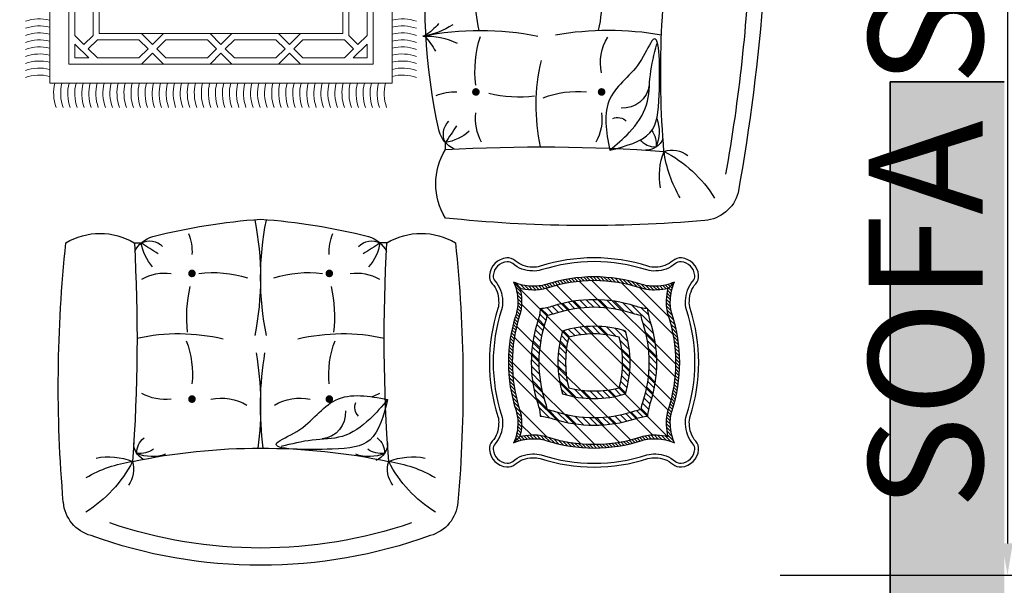
# Model space of a CAD drawing. Units: inches. Extents: x 3592 to 4861, y 1650 to 2243.
# Tile 5 of 30: x 4188 to 4265, y 1872 to 1916. Entities that reach past the tile are written whole.
import ezdxf

# ---------------------------------------------------------------- set-up
doc = ezdxf.new("R2010")
doc.units = ezdxf.units.IN
for name, color, linetype, lineweight in [('A-ANNO-DIMS', 2, 'Continuous', 13), ('A-FURN', 9, 'Continuous', 13), ('A-WALL', 7, 'Continuous', 35), ('RA-AP-01$0$INT', 35, 'Continuous', 5)]:
    doc.layers.add(name, color=color, linetype=linetype, lineweight=lineweight)
doc.layers.add('A-WALL-PATT', color=252, linetype='Continuous', lineweight=13, true_color=0x939598)
for name, color, linetype in [('RA-AP-01$0$FURN', 3, 'Continuous'), ('RA-AP-01$0$WOOD', 64, 'Continuous'), ('RA-AP-02$0$FLPT', 30, 'Continuous')]:
    doc.layers.add(name, color=color, linetype=linetype)
doc.styles.get("Standard").update_dxf_attribs({"font": 'arial.ttf'})
doc.dimstyles.new('ISO-25', dxfattribs={"dimtxt": 9, "dimasz": 2.5, "dimexe": 1.25, "dimexo": 0.625, "dimtad": 1, "dimlunit": 3, "dimtxsty": 'Standard', "dimcen": 2.5, "dimadec": 0, "dimazin": 0, "dimtfac": 1, "dimtmove": 0, "dimatfit": 3, "dimfxl": 1, "dimarcsym": 0})
pattern_1 = [(225, (10.907943, -14.206733), (0.008838835, -0.008838835), [])]
pattern_2 = [(225, (10.9079426, -14.206733), (0.0044194174, -0.0044194174), [])]

# ---------------------------------------------------------------- blocks, each defined once
blk = doc.blocks.new('A$C7F4351E2')
at = {"layer": 'RA-AP-01$0$FURN'}
for p, q in [((8.3526, -8.2639), (8.3526, -8.2823)), ((8.3526, -8.9277), (8.3526, -8.9094))]:
    blk.add_line(p, q, dxfattribs=at)
at = {"layer": 'RA-AP-01$0$FURN', "const_width": 0.01}
for points in [[(8.4378, -8.4154, 1), (8.4278, -8.4154, 1)], [(8.7582, -8.4154, -1), (8.7682, -8.4154, -1)], [(8.4378, -8.7763, -1), (8.4278, -8.7763, -1)], [(8.7582, -8.7763, 1), (8.7682, -8.7763, 1)]]:
    blk.add_lwpolyline(points, format="xyb", close=True, dxfattribs=at)
at = {"layer": 'RA-AP-01$0$FURN'}
for centre, radius, start, end in [((8.7276, -11.6169), 3.5528, 85.0473, 96.0589), ((8.5021, -8.1739), 0.1745, 148.9518, 211.0482), ((9.0257, -8.177), 0.1, 15.4995, 85.0473), ((8.7725, -7.9585), 0.3382, 297.2303, 328.2564), ((9.2485, -8.3027), 0.3242, 149.2986, 172.3026), ((7.8898, -8.5958), 1.3103, 340.1193, 19.8807), ((9.0849, -8.196), 0.1699, 168.8778, 201.8512), ((7.9299, -8.5958), 1.2249, 341.1257, 18.8743), ((8.9477, -8.1918), 0.0705, 253.1339, 306.4126), ((8.4085, -8.333), 0.0754, 115.8746, 163.9834), ((8.6036, -3.7971), 4.4739, 266.7829, 274.1477), ((9.1012, -8.3803), 0.5101, 167.6182, 193.3122), ((8.9033, -8.3184), 0.0479, 86.5753, 142.6834), ((8.8784, -8.3122), 0.05, 30.1478, 90), ((10.5271, -8.5958), 1.6349, 168.12, 191.88), ((8.8381, -8.2768), 0.0683, 326.673, 5.2184), ((8.8101, -8.3111), 0.1042, 340.4828, 22.8693), ((8.3954, -8.3042), 0.0479, 152.8071, 225.4025), ((8.3336, -8.4027), 0.1219, 48.0376, 81.0462), ((7.4396, -8.9138), 1.1102, 31.9329, 34.6665), ((8.5531, -8.3441), 0.1214, 150.1419, 187.6917), ((8.6429, -8.3441), 0.1214, 352.3083, 29.8581), ((9.8263, -8.6967), 1.5391, 165.5339, 176.2438), ((8.3749, -8.2943), 0.1213, 247.3376, 273.7315), ((8.547, -8.7534), 0.3517, 83.4125, 103.1675), ((8.6977, -8.1725), 0.2442, 248.9017, 275.9924), ((8.7329, -8.4698), 0.3024, 173.0945, 197.5881), ((8.8899, -8.4923), 0.1295, 167.9901, 211.3796), ((8.4441, -7.8299), 0.7655, 258.6273, 281.4174), ((8.7812, -7.7726), 0.8233, 260.2449, 277.7495), ((9.8263, -8.495), 1.5391, 183.7562, 194.4661), ((8.4441, -9.3613), 0.7655, 78.5826, 101.3727), ((8.7812, -9.4187), 0.8233, 82.2506, 99.7551), ((8.7329, -8.7219), 0.3024, 162.4119, 186.9055), ((8.8899, -8.6994), 0.1295, 148.6204, 192.0099), ((9.1012, -8.8113), 0.5101, 166.6878, 192.3818), ((8.7996, -8.75), 0.0689, 265.5384, 353.5805), ((8.3749, -8.8974), 0.1213, 86.2685, 112.6624), ((8.547, -8.4383), 0.3517, 256.8325, 276.5875), ((8.6977, -9.0192), 0.2442, 84.0076, 111.0983), ((8.5531, -8.8476), 0.1214, 172.3083, 209.8581), ((8.7851, -8.8743), 0.031, 42.6211, 114.224), ((8.8101, -8.8806), 0.1042, 337.1307, 19.5172), ((8.3954, -8.8875), 0.0479, 134.5975, 207.1929), ((7.4396, -8.2779), 1.1102, 325.3335, 328.0671), ((8.4085, -8.8587), 0.0754, 196.0166, 244.1254), ((8.3336, -8.789), 0.1219, 278.9538, 311.9624), ((8.6429, -8.8476), 0.1214, 330.1419, 340.3914), ((8.8784, -8.8795), 0.05, 270, 337.4173), ((8.8381, -8.9149), 0.0683, 354.7816, 33.327), ((8.6036, -13.3946), 4.4739, 85.8523, 93.2171), ((8.9033, -8.8733), 0.0479, 217.3166, 273.4247), ((8.5021, -9.0177), 0.1745, 148.9518, 211.0482), ((9.0849, -8.9957), 0.1699, 158.1488, 191.1222), ((8.9477, -8.9999), 0.0705, 53.5874, 106.8661), ((8.7725, -9.2331), 0.3382, 31.7436, 62.7697), ((9.2485, -8.889), 0.3242, 187.6974, 210.7014), ((9.0257, -9.0147), 0.1, 274.9527, 344.5005), ((8.7276, -5.5748), 3.5528, 263.9411, 274.9527)]:
    blk.add_arc(centre, radius, start, end, dxfattribs=at)
for points, knots in [([(8.7644, -8.9296), (8.7553, -8.8811), (8.742, -8.8109), (8.806, -8.7405), (8.8475, -8.7011), (8.8971, -8.5832), (8.8971, -8.7848), (8.8861, -8.8978), (8.8065, -8.9186), (8.7644, -8.9296)], [0, 0, 0, 0, 0.1367587, 0.1981302, 0.267773, 0.3281195, 0.4737578, 0.5765194, 0.6920332, 0.6920332, 0.6920332, 0.6920332]), ([(8.7644, -8.9296), (8.7822, -8.9146), (8.8216, -8.8815), (8.8692, -8.8143), (8.8678, -8.7293), (8.8812, -8.6768), (8.8881, -8.6498)], [0, 0, 0, 0, 0.0700185, 0.155078, 0.2344492, 0.3178049, 0.3178049, 0.3178049, 0.3178049])]:
    blk.add_open_spline(points, degree=3, knots=knots, dxfattribs=at)
blk = doc.blocks.new('A$C67D63ADA')
at = {"layer": 'RA-AP-01$0$INT'}
for p, q in [((5.4297, -6.2594), (5.5219, -6.2594)), ((5.5219, -6.2594), (5.5459, -6.2834)), ((5.5446, -6.2594), (5.5812, -6.2594)), ((5.5812, -6.2961), (5.5446, -6.2594)), ((5.5812, -6.2961), (5.5812, -6.2594)), ((5.5219, -6.3074), (5.5459, -6.2834)), ((5.5219, -6.3074), (5.4297, -6.3074)), ((5.5332, -6.3187), (5.5572, -6.2947)), ((5.5812, -6.3187), (5.5572, -6.2947)), ((5.5332, -6.4281), (5.5332, -6.3187)), ((5.5812, -6.4281), (5.5812, -6.3187)), ((5.5172, -6.3538), (5.5172, -6.933)), ((5.5172, -6.3538), (5.5172, -6.933)), ((5.5172, -6.4347), (5.5459, -6.4634)), ((5.5332, -6.4281), (5.5572, -6.4521)), ((5.5812, -6.4281), (5.5572, -6.4521)), ((5.5972, -6.4347), (5.5686, -6.4634)), ((5.5172, -6.4921), (5.5459, -6.4634)), ((5.5972, -6.4921), (5.5686, -6.4634)), ((5.5332, -6.4987), (5.5572, -6.4747)), ((5.5812, -6.4987), (5.5572, -6.4747)), ((5.5332, -6.6081), (5.5332, -6.4987)), ((5.5812, -6.6081), (5.5812, -6.4987)), ((5.5172, -6.6147), (5.5459, -6.6434)), ((5.5332, -6.6081), (5.5572, -6.6321)), ((5.5812, -6.6081), (5.5572, -6.6321)), ((5.5972, -6.6147), (5.5686, -6.6434)), ((5.5172, -6.6721), (5.5459, -6.6434)), ((5.5972, -6.6721), (5.5686, -6.6434)), ((5.5332, -6.6787), (5.5572, -6.6547)), ((5.5812, -6.6787), (5.5572, -6.6547)), ((5.5332, -6.6787), (5.5332, -6.7881)), ((5.5812, -6.6787), (5.5812, -6.7881)), ((5.5172, -6.7947), (5.5459, -6.8234)), ((5.5332, -6.7881), (5.5572, -6.8121)), ((5.5812, -6.7881), (5.5572, -6.8121)), ((5.5972, -6.7947), (5.5686, -6.8234)), ((5.5172, -6.8521), (5.5459, -6.8234)), ((5.5972, -6.8521), (5.5686, -6.8234)), ((5.5332, -6.8587), (5.5572, -6.8347)), ((5.5812, -6.8587), (5.5572, -6.8347)), ((5.5332, -6.8587), (5.5332, -6.9681)), ((5.5812, -6.8587), (5.5812, -6.9681)), ((5.5219, -6.9794), (5.4297, -6.9794)), ((5.5219, -6.9794), (5.5459, -7.0034)), ((5.5332, -6.9681), (5.5572, -6.9921)), ((5.5812, -6.9681), (5.5572, -6.9921)), ((5.5219, -7.0274), (5.5459, -7.0034)), ((5.5812, -6.9907), (5.5446, -7.0274)), ((5.5812, -6.9907), (5.5812, -7.0274)), ((5.4297, -7.0274), (5.5219, -7.0274)), ((5.5446, -7.0274), (5.5812, -7.0274))]:
    blk.add_line(p, q, dxfattribs=at)
for points in [[(5.6472, -6.2434), (5.6472, -7.0934), (4.1072, -7.0934), (4.1072, -6.1934), (4.8772, -6.1934)], [(4.8772, -6.1934), (5.6472, -6.1934), (5.6472, -7.0934), (4.8772, -7.0934)], [(5.5972, -6.2434), (5.5972, -7.0434), (4.1572, -7.0434), (4.1572, -6.2434)], [(4.8772, -6.2434), (5.5972, -6.2434)], [(4.8772, -6.3234), (5.5172, -6.3234), (5.5172, -6.9634), (4.8772, -6.9634)]]:
    blk.add_lwpolyline(points, dxfattribs=at)
for centre, start, end in [((5.5875, -6.1665), 160.2038, 194.3025), ((5.606, -6.1665), 160.2038, 194.3025), ((5.6245, -6.1665), 160.2038, 194.3025), ((5.643, -6.1665), 160.2038, 194.3025), ((5.6614, -6.1665), 160.2038, 194.3025), ((5.6799, -6.1665), 160.2038, 194.3025), ((5.6984, -6.1665), 160.2038, 194.3025), ((5.7169, -6.1665), 160.2038, 194.3025), ((5.7354, -6.1665), 160.2038, 194.3025), ((5.6742, -6.1053), 255.6975, 289.7962), ((5.6742, -6.1238), 255.6975, 289.7962), ((5.6742, -6.1423), 255.6975, 289.7962), ((5.6742, -6.1607), 255.6975, 289.7962), ((5.6742, -6.1792), 255.6975, 289.7962), ((5.6742, -6.1977), 255.6975, 289.7962), ((5.6742, -6.2162), 255.6975, 289.7962), ((5.6742, -6.2347), 255.6975, 289.7962), ((5.6742, -6.2531), 255.6975, 289.7962), ((5.6742, -6.2716), 255.6975, 289.7962), ((5.6742, -6.2901), 255.6975, 289.7962), ((5.6742, -6.3086), 255.6975, 289.7962), ((5.6742, -6.3271), 255.6975, 289.7962), ((5.6742, -6.3455), 255.6975, 289.7962), ((5.6742, -6.364), 255.6975, 289.7962), ((5.6742, -6.3825), 255.6975, 289.7962), ((5.6742, -6.401), 255.6975, 289.7962), ((5.6742, -6.4195), 255.6975, 289.7962), ((5.6742, -6.4379), 255.6975, 289.7962), ((5.6742, -6.4564), 255.6975, 289.7962), ((5.6742, -6.4749), 255.6975, 289.7962), ((5.6742, -6.4934), 255.6975, 289.7962), ((5.6742, -6.5119), 255.6975, 289.7962), ((5.6742, -6.5303), 255.6975, 289.7962), ((5.6742, -6.5488), 255.6975, 289.7962), ((5.6742, -6.5673), 255.6975, 289.7962), ((5.6742, -6.5858), 255.6975, 289.7962), ((5.6742, -6.6043), 255.6975, 289.7962), ((5.6742, -6.6227), 255.6975, 289.7962), ((5.6742, -6.6412), 255.6975, 289.7962), ((5.6742, -6.6597), 255.6975, 289.7962), ((5.6742, -6.6782), 255.6975, 289.7962), ((5.6742, -6.6967), 255.6975, 289.7962), ((5.6742, -6.7151), 255.6975, 289.7962), ((5.6742, -6.7336), 255.6975, 289.7962), ((5.6742, -6.7521), 255.6975, 289.7962), ((5.6742, -6.7706), 255.6975, 289.7962), ((5.6742, -6.7891), 255.6975, 289.7962), ((5.6742, -6.8075), 255.6975, 289.7962), ((5.6742, -6.826), 255.6975, 289.7962), ((5.6742, -6.8445), 255.6975, 289.7962), ((5.6742, -6.863), 255.6975, 289.7962), ((5.6742, -6.8815), 255.6975, 289.7962), ((5.6742, -6.8999), 255.6975, 289.7962), ((5.6742, -6.9184), 255.6975, 289.7962), ((5.6742, -6.9369), 255.6975, 289.7962), ((5.6742, -6.9554), 255.6975, 289.7962), ((5.6742, -6.9739), 255.6975, 289.7962), ((5.5875, -7.1204), 165.6975, 199.7962), ((5.606, -7.1204), 165.6975, 199.7962), ((5.6245, -7.1204), 165.6975, 199.7962), ((5.643, -7.1204), 165.6975, 199.7962), ((5.6614, -7.1204), 165.6975, 199.7962), ((5.6799, -7.1204), 165.6975, 199.7962), ((5.6984, -7.1204), 165.6975, 199.7962), ((5.7169, -7.1204), 165.6975, 199.7962), ((5.7354, -7.1204), 165.6975, 199.7962)]:
    blk.add_arc(centre, 0.1091, start, end, dxfattribs=at)
blk = doc.blocks.new('A$C7EE91E48')
at = {"layer": 'RA-AP-01$0$FURN'}
blk.add_line((9.7755, -8.9166), (9.7571, -8.9166), dxfattribs=at)
at = {"layer": 'RA-AP-01$0$FURN', "const_width": 0.01}
for points in [[(9.624, -9.0019, 1), (9.624, -8.9919, 1)], [(9.624, -9.3223, -1), (9.624, -9.3323, -1)]]:
    blk.add_lwpolyline(points, format="xyb", close=True, dxfattribs=at)
at = {"layer": 'RA-AP-01$0$FURN'}
for centre, radius, start, end in [((9.3879, -10.4424), 1.5791, 77.592, 96.5884), ((9.3421, -8.7788), 0.1579, 310.3865, 328.0658), ((9.2924, -8.8326), 0.1864, 326.2926, 352.3818), ((10.2276, -9.0082), 0.7655, 168.6273, 191.4174), ((9.6686, -8.8653), 0.1916, 177.5853, 205.5831), ((9.5886, -8.7497), 0.1579, 225.4052, 243.0845), ((9.7451, -8.939), 0.1213, 157.3376, 183.7315), ((9.7064, -8.9726), 0.0754, 25.8746, 73.9834), ((9.8655, -9.0661), 0.1745, 58.9518, 121.0482), ((9.7352, -8.9594), 0.0479, 62.8071, 135.4025), ((9.1256, -8.0037), 1.1102, 301.9329, 304.6665), ((9.6367, -8.8976), 0.1219, 318.0376, 351.0462), ((14.2423, -9.1677), 4.4739, 176.7829, 184.1477), ((6.4225, -9.2916), 3.5528, 355.0473, 6.0589), ((9.3827, -9.3452), 0.3487, 76.8392, 92.4658), ((9.5696, -9.2969), 0.3024, 83.0945, 107.5881), ((9.6953, -9.1172), 0.1214, 60.1419, 97.6917), ((9.286, -9.111), 0.3517, 353.4125, 13.1675), ((9.6591, -9.6653), 0.5101, 77.6182, 103.3122), ((9.8669, -9.2618), 0.2442, 158.9017, 185.9924), ((10.285, -9.3453), 0.8233, 170.2449, 189.7551), ((9.6953, -9.2069), 0.1214, 262.3083, 299.8581), ((9.3827, -8.9789), 0.3487, 267.5342, 283.1608), ((9.5471, -9.4539), 0.1295, 77.9901, 121.3796), ((9.722, -9.3692), 0.031, 155.776, 227.3789), ((9.5977, -9.3837), 0.0689, 276.4195, 4.4616), ((9.7272, -9.4424), 0.05, 292.5827, 360), ((9.721, -9.4673), 0.0479, 356.5753, 52.6834), ((9.7626, -9.4022), 0.0683, 236.673, 275.2184), ((9.5748, -11.9348), 2.4522, 85.1961, 99.8458), ((9.7283, -9.3742), 0.1042, 250.4828, 292.8693), ((9.8476, -9.5117), 0.0705, 163.1339, 216.4126), ((9.8434, -9.649), 0.1699, 78.8778, 111.8512), ((9.7367, -9.8125), 0.3242, 59.2986, 82.3026), ((10.0809, -9.3365), 0.3382, 207.2303, 238.2564), ((9.8624, -9.5897), 0.1, 285.4995, 355.0473), ((9.0796, -5.4361), 4.2848, 272.1916, 280.2199), ((8.936, -4.2841), 5.4854, 268.8504, 280.0061)]:
    blk.add_arc(centre, radius, start, end, dxfattribs=at)
for points, knots in [([(9.7773, -9.3485), (9.7288, -9.3393), (9.6586, -9.326), (9.5882, -9.3901), (9.5488, -9.4315), (9.4309, -9.4812), (9.6325, -9.4811), (9.7455, -9.4702), (9.7663, -9.3906), (9.7773, -9.3485)], [0, 0, 0, 0, 0.1367587, 0.1981302, 0.267773, 0.3281195, 0.4737578, 0.5765194, 0.6920332, 0.6920332, 0.6920332, 0.6920332]), ([(9.7773, -9.3485), (9.7623, -9.3663), (9.7292, -9.4056), (9.662, -9.4532), (9.577, -9.4519), (9.5245, -9.4653), (9.4975, -9.4722)], [0, 0, 0, 0, 0.0700185, 0.155078, 0.2344492, 0.3178049, 0.3178049, 0.3178049, 0.3178049])]:
    blk.add_open_spline(points, degree=3, knots=knots, dxfattribs=at)
blk = doc.blocks.new('A$C3E710961')
at = {"layer": 'RA-AP-01$0$WOOD'}
h = blk.add_hatch(dxfattribs=at)
h.set_pattern_fill('ANSI31', color=256, scale=0.05, angle=180, style=0)
h.set_pattern_definition(pattern_2)
h.paths.add_polyline_path([(5.8026, -7.4494, 0.094014), (5.8075, -7.4087, 0.060627), (5.8033, -7.3781, 0.060627), (5.8339, -7.3823, 0.094014), (5.8746, -7.3774, -0.130533), (6.0799, -7.3664), (6.0868, -7.3576, 0.133623), (5.8716, -7.3679, -0.094597), (5.8343, -7.3723, -0.104317), (5.7868, -7.3616, -0.104317), (5.7975, -7.4091, -0.094597), (5.7931, -7.4464, 0.158024), (5.7931, -7.6995, -0.094597), (5.7975, -7.7367, -0.104317), (5.7868, -7.7842, -0.104317), (5.8343, -7.7736, -0.094597), (5.8716, -7.778, 0.158024), (6.1247, -7.778, -0.094597), (6.1619, -7.7736, -0.104317), (6.2094, -7.7842, -0.104317), (6.1987, -7.7367, -0.094597), (6.2031, -7.6995, 0.158024), (6.2031, -7.4464, -0.094597), (6.1987, -7.4091, -0.104317), (6.2094, -7.3616, -0.104317), (6.1619, -7.3723, -0.094597), (6.1247, -7.3679, 0.023897), (6.0868, -7.3576), (6.0799, -7.3664, -0.026981), (6.1216, -7.3774, 0.094014), (6.1623, -7.3823, 0.060627), (6.193, -7.3781, 0.060627), (6.1888, -7.4087, 0.094014), (6.1936, -7.4494, -0.158071), (6.1936, -7.6964, 0.094014), (6.1888, -7.7372, 0.060627), (6.193, -7.7678, 0.060627), (6.1623, -7.7636, 0.094014), (6.1216, -7.7684, -0.158071), (5.8746, -7.7684, 0.094014), (5.8339, -7.7636, 0.060627), (5.8033, -7.7678, 0.060627), (5.8075, -7.7372, 0.094014), (5.8026, -7.6964, -0.158071)])
h = blk.add_hatch(dxfattribs=at)
h.set_pattern_fill('ANSI31', color=256, scale=0.05, angle=180, style=0)
h.set_pattern_definition(pattern_2)
h.paths.add_polyline_path([(5.8026, -7.4494, 0.094014), (5.8075, -7.4087, 0.060627), (5.8033, -7.3781, 0.060627), (5.8339, -7.3823, 0.094014), (5.8746, -7.3774, -0.130533), (6.0799, -7.3664), (6.0868, -7.3576, 0.133623), (5.8716, -7.3679, -0.094597), (5.8343, -7.3723, -0.104317), (5.7868, -7.3616, -0.104317), (5.7975, -7.4091, -0.094597), (5.7931, -7.4464, 0.158024), (5.7931, -7.6995, -0.094597), (5.7975, -7.7367, -0.104317), (5.7868, -7.7842, -0.104317), (5.8343, -7.7736, -0.094597), (5.8716, -7.778, 0.158024), (6.1247, -7.778, -0.094597), (6.1619, -7.7736, -0.104317), (6.2094, -7.7842, -0.104317), (6.1987, -7.7367, -0.094597), (6.2031, -7.6995, 0.158024), (6.2031, -7.4464, -0.094597), (6.1987, -7.4091, -0.104317), (6.2094, -7.3616, -0.104317), (6.1619, -7.3723, -0.094597), (6.1247, -7.3679, 0.023897), (6.0868, -7.3576), (6.0799, -7.3664, -0.026981), (6.1216, -7.3774, 0.094014), (6.1623, -7.3823, 0.060627), (6.193, -7.3781, 0.060627), (6.1888, -7.4087, 0.094014), (6.1936, -7.4494, -0.158071), (6.1936, -7.6964, 0.094014), (6.1888, -7.7372, 0.060627), (6.193, -7.7678, 0.060627), (6.1623, -7.7636, 0.094014), (6.1216, -7.7684, -0.158071), (5.8746, -7.7684, 0.094014), (5.8339, -7.7636, 0.060627), (5.8033, -7.7678, 0.060627), (5.8075, -7.7372, 0.094014), (5.8026, -7.6964, -0.158071)])
h = blk.add_hatch(dxfattribs=at)
h.set_pattern_fill('ANSI32,_I', color=256, scale=0.2, angle=180, style=2)
h.set_pattern_definition([(225, (-0.32707, -3.57881), (0.053033, -0.053033), []), (225, (-0.36242, -3.57881), (0.053033, -0.053033), [])])
h.paths.add_polyline_path([(5.8693, -7.675, -0.030626), (5.8746, -7.6964, -0.030626), (5.896, -7.7018, 0.158398), (6.1002, -7.7018, -0.030626), (6.1216, -7.6964, -0.030626), (6.127, -7.675, 0.158398), (6.127, -7.4708, -0.030626), (6.1216, -7.4495, -0.030626), (6.1002, -7.4441, 0.158398), (5.896, -7.4441, -0.030626), (5.8746, -7.4495, -0.030626), (5.8693, -7.4708, 0.158398)], flags=16)
h.paths.add_polyline_path([(5.8026, -7.6964, -0.094014), (5.8075, -7.7372, -0.060627), (5.8033, -7.7678, -0.060627), (5.8339, -7.7636, -0.094014), (5.8746, -7.7684, 0.158071), (6.1216, -7.7684, -0.094014), (6.1623, -7.7636, -0.060627), (6.193, -7.7678, -0.060627), (6.1888, -7.7372, -0.094014), (6.1936, -7.6964, 0.158071), (6.1936, -7.4494, -0.094014), (6.1888, -7.4087, -0.060627), (6.193, -7.3781, -0.060627), (6.1623, -7.3823, -0.094014), (6.1216, -7.3774, 0.158071), (5.8746, -7.3774, -0.094014), (5.8339, -7.3823, -0.060627), (5.8033, -7.3781, -0.060627), (5.8075, -7.4087, -0.094014), (5.8026, -7.4494, 0.158071)])
h.paths.add_polyline_path([(5.8693, -7.4708, 0.030626), (5.8746, -7.4495, 0.030626), (5.896, -7.4441, -0.158398), (6.1002, -7.4441, 0.030626), (6.1216, -7.4495, 0.030626), (6.127, -7.4708, -0.158398), (6.127, -7.675, 0.030626), (6.1216, -7.6964, 0.030626), (6.1002, -7.7018, -0.158398), (5.896, -7.7018, 0.030626), (5.8746, -7.6964, 0.030626), (5.8693, -7.675, -0.158398)], flags=0)
h = blk.add_hatch(dxfattribs=at)
h.set_pattern_fill('ANSI31', color=256, scale=0.1, angle=180, style=0)
h.set_pattern_definition(pattern_1)
h.paths.add_polyline_path([(5.8693, -7.675, -0.158398), (5.8693, -7.4708, 0.030626), (5.8746, -7.4495, 0.030626), (5.896, -7.4441, -0.102814), (6.0297, -7.4294), (6.0443, -7.411, 0.112048), (5.8899, -7.425, -0.052642), (5.857, -7.4318, -0.052642), (5.8502, -7.4647, 0.158303), (5.8502, -7.6812, -0.052642), (5.857, -7.7141, -0.052642), (5.8899, -7.7208, 0.0216), (5.919, -7.7289), (5.9329, -7.7115, -0.028915), (5.896, -7.7018, 0.030626), (5.8746, -7.6964, 0.030626)])
h.paths.add_polyline_path([(5.9329, -7.7115), (5.919, -7.7289, 0.136237), (6.1063, -7.7208, -0.052642), (6.1392, -7.7141, -0.052642), (6.146, -7.6812, 0.158303), (6.146, -7.4647, -0.052642), (6.1392, -7.4318, -0.052642), (6.1063, -7.425, 0.045448), (6.0443, -7.411), (6.0297, -7.4294, -0.054693), (6.1002, -7.4441, 0.030626), (6.1216, -7.4495, 0.030626), (6.127, -7.4708, -0.158398), (6.127, -7.675, 0.030626), (6.1216, -7.6964, 0.030626), (6.1002, -7.7018, -0.128893)])
h.paths.add_polyline_path([(6.0645, -7.6394, -0.078369), (5.9838, -7.6476), (5.9688, -7.6664, 0.101268), (6.0807, -7.6555, 0.125365), (6.0875, -7.5173), (6.0708, -7.5383, -0.098159)], flags=17)
h.paths.add_polyline_path([(6.0645, -7.5065, -0.031109), (6.0708, -7.5383), (6.0875, -7.5173, 0.024773), (6.0807, -7.4904, 0.081275), (5.991, -7.478), (5.9743, -7.499, -0.087626)], flags=17)
h.paths.add_polyline_path([(5.9155, -7.4904, 0.150605), (5.9155, -7.6555, 0.048597), (5.9688, -7.6664), (5.9838, -7.6476, -0.05078), (5.9317, -7.6394, -0.129665), (5.9317, -7.5065, -0.041567), (5.9743, -7.499), (5.991, -7.478, 0.068492)], flags=17)
h = blk.add_hatch(dxfattribs=at)
h.set_pattern_fill('ANSI31', color=256, scale=0.1, angle=180, style=0)
h.set_pattern_definition(pattern_1)
h.paths.add_polyline_path([(5.8693, -7.675, -0.158398), (5.8693, -7.4708, 0.030626), (5.8746, -7.4495, 0.030626), (5.896, -7.4441, -0.102814), (6.0297, -7.4294), (6.0443, -7.411, 0.112048), (5.8899, -7.425, -0.052642), (5.857, -7.4318, -0.052642), (5.8502, -7.4647, 0.158303), (5.8502, -7.6812, -0.052642), (5.857, -7.7141, -0.052642), (5.8899, -7.7208, 0.0216), (5.919, -7.7289), (5.9329, -7.7115, -0.028915), (5.896, -7.7018, 0.030626), (5.8746, -7.6964, 0.030626)])
h.paths.add_polyline_path([(5.9329, -7.7115), (5.919, -7.7289, 0.136237), (6.1063, -7.7208, -0.052642), (6.1392, -7.7141, -0.052642), (6.146, -7.6812, 0.158303), (6.146, -7.4647, -0.052642), (6.1392, -7.4318, -0.052642), (6.1063, -7.425, 0.045448), (6.0443, -7.411), (6.0297, -7.4294, -0.054693), (6.1002, -7.4441, 0.030626), (6.1216, -7.4495, 0.030626), (6.127, -7.4708, -0.158398), (6.127, -7.675, 0.030626), (6.1216, -7.6964, 0.030626), (6.1002, -7.7018, -0.128893)])
h.paths.add_polyline_path([(6.0645, -7.6394, -0.078369), (5.9838, -7.6476), (5.9688, -7.6664, 0.101268), (6.0807, -7.6555, 0.125365), (6.0875, -7.5173), (6.0708, -7.5383, -0.098159)], flags=17)
h.paths.add_polyline_path([(6.0645, -7.5065, -0.031109), (6.0708, -7.5383), (6.0875, -7.5173, 0.024773), (6.0807, -7.4904, 0.081275), (5.991, -7.478), (5.9743, -7.499, -0.087626)], flags=17)
h.paths.add_polyline_path([(5.9155, -7.4904, 0.150605), (5.9155, -7.6555, 0.048597), (5.9688, -7.6664), (5.9838, -7.6476, -0.05078), (5.9317, -7.6394, -0.129665), (5.9317, -7.5065, -0.041567), (5.9743, -7.499), (5.991, -7.478, 0.068492)], flags=17)
for p, q in [((5.8033, -7.3781), (5.7868, -7.3616)), ((5.8033, -7.3781), (5.7868, -7.3616)), ((5.8033, -7.7678), (5.7868, -7.7842)), ((5.8033, -7.7678), (5.7868, -7.7842)), ((6.193, -7.7678), (6.2094, -7.7842)), ((6.193, -7.7678), (6.2094, -7.7842))]:
    blk.add_line(p, q, dxfattribs=at)
for points in [[(6.2052, -7.8404, 0.205661), (6.2277, -7.8477, 0.361434), (6.2729, -7.8025, 0.205661), (6.2656, -7.78, -0.184266), (6.2487, -7.7346, -0.100949), (6.2508, -7.7147, 0.157773), (6.2508, -7.4312, -0.100949), (6.2487, -7.4113, -0.184266), (6.2656, -7.3659, 0.205661), (6.2729, -7.3434, 0.361434), (6.2277, -7.2981, 0.205661), (6.2052, -7.3055, -0.184266), (6.1597, -7.3223, -0.100949), (6.1399, -7.3203, 0.157773), (5.8564, -7.3203, -0.100949), (5.8365, -7.3223, -0.184266), (5.791, -7.3055, 0.205661), (5.7685, -7.2981, 0.361434), (5.7233, -7.3434, 0.205661), (5.7306, -7.3659, -0.184266), (5.7475, -7.4113, -0.100949), (5.7454, -7.4312, 0.157773), (5.7454, -7.7147, -0.100949), (5.7475, -7.7346, -0.184266), (5.7306, -7.78, 0.205661), (5.7233, -7.8025, 0.361434), (5.7685, -7.8477, 0.205661), (5.791, -7.8404, -0.184266), (5.8365, -7.8236, -0.100949), (5.8564, -7.8256, 0.157773), (6.1399, -7.8256, -0.100949), (6.1597, -7.8236, -0.184266)], [(6.2118, -7.8329, 0.205661), (6.2268, -7.8378, 0.361434), (6.2629, -7.8016, 0.205661), (6.2581, -7.7866, -0.182482), (6.2387, -7.735, -0.098854), (6.2412, -7.7117, 0.157827), (6.2412, -7.4342, -0.098854), (6.2387, -7.4109, -0.182482), (6.2581, -7.3593, 0.205661), (6.2629, -7.3443, 0.361434), (6.2268, -7.3081, 0.205661), (6.2118, -7.313, -0.182482), (6.1602, -7.3323, -0.098854), (6.1368, -7.3298, 0.157827), (5.8594, -7.3298, -0.098854), (5.836, -7.3323, -0.182482), (5.7845, -7.313, 0.205661), (5.7694, -7.3081, 0.361434), (5.7333, -7.3443, 0.205661), (5.7382, -7.3593, -0.182482), (5.7575, -7.4109, -0.098854), (5.755, -7.4342, 0.157827), (5.755, -7.7117, -0.098854), (5.7575, -7.735, -0.182482), (5.7382, -7.7866, 0.205661), (5.7333, -7.8016, 0.361434), (5.7694, -7.8378, 0.205661), (5.7845, -7.8329, -0.182482), (5.836, -7.8136, -0.098854), (5.8594, -7.8161, 0.157827), (6.1368, -7.8161, -0.098854), (6.1602, -7.8136, -0.182482)], [(6.2094, -7.7842, -0.104317), (6.1987, -7.7367, -0.094597), (6.2031, -7.6995, 0.158024), (6.2031, -7.4464, -0.094597), (6.1987, -7.4091, -0.104317), (6.2094, -7.3616, -0.104317), (6.1619, -7.3723, -0.094597), (6.1247, -7.3679, 0.158024), (5.8716, -7.3679, -0.094597), (5.8343, -7.3723, -0.104317), (5.7868, -7.3616, -0.104317), (5.7975, -7.4091, -0.094597), (5.7931, -7.4464, 0.158024), (5.7931, -7.6995, -0.094597), (5.7975, -7.7367, -0.104317), (5.7868, -7.7842, -0.104317), (5.8343, -7.7736, -0.094597), (5.8716, -7.778, 0.158024), (6.1247, -7.778, -0.094597), (6.1619, -7.7736, -0.104317)], [(6.193, -7.7678, -0.060627), (6.1888, -7.7372, -0.094014), (6.1936, -7.6964, 0.158071), (6.1936, -7.4494, -0.094014), (6.1888, -7.4087, -0.060627), (6.193, -7.3781, -0.060627), (6.1623, -7.3823, -0.094014), (6.1216, -7.3774, 0.158071), (5.8746, -7.3774, -0.094014), (5.8339, -7.3823, -0.060627), (5.8033, -7.3781, -0.060627), (5.8075, -7.4087, -0.094014), (5.8026, -7.4494, 0.158071), (5.8026, -7.6964, -0.094014), (5.8075, -7.7372, -0.060627), (5.8033, -7.7678, -0.060627), (5.8339, -7.7636, -0.094014), (5.8746, -7.7684, 0.158071), (6.1216, -7.7684, -0.094014), (6.1623, -7.7636, -0.060627)], [(6.1392, -7.7141, -0.052642), (6.146, -7.6812, 0.158303), (6.146, -7.4647, -0.052642), (6.1392, -7.4318, -0.052642), (6.1063, -7.425, 0.158303), (5.8899, -7.425, -0.052642), (5.857, -7.4318, -0.052642), (5.8502, -7.4647, 0.158303), (5.8502, -7.6812, -0.052642), (5.857, -7.7141, -0.052642), (5.8899, -7.7208, 0.158303), (6.1063, -7.7208, -0.052642)], [(6.1216, -7.6964, -0.030626), (6.127, -7.675, 0.158398), (6.127, -7.4708, -0.030626), (6.1216, -7.4495, -0.030626), (6.1002, -7.4441, 0.158398), (5.896, -7.4441, -0.030626), (5.8746, -7.4495, -0.030626), (5.8693, -7.4708, 0.158398), (5.8693, -7.675, -0.030626), (5.8746, -7.6964, -0.030626), (5.896, -7.7018, 0.158398), (6.1002, -7.7018, -0.030626)], [(6.0807, -7.6555, 0.150605), (6.0807, -7.4904, 0.150605), (5.9155, -7.4904, 0.150605), (5.9155, -7.6555, 0.150605)], [(6.0645, -7.6394, 0.129665), (6.0645, -7.5065, 0.129665), (5.9317, -7.5065, 0.129665), (5.9317, -7.6394, 0.129665)]]:
    blk.add_lwpolyline(points, format="xyb", close=True, dxfattribs=at)
blk = doc.blocks.new('A$C44E37296')
at = {"layer": 'RA-AP-01$0$FURN'}
blk.add_blockref('A$C3E710961', (-4.4617, 9.3428), dxfattribs=at)
at = {"layer": 'RA-AP-01$0$WOOD', "xscale": -1, "rotation": 180}
for name, p in [('A$C7EE91E48', (-8.7987, -7.5375)), ('A$C7F4351E2', (-7.1305, -7.7021))]:
    blk.add_blockref(name, p, dxfattribs=at)
at = {"layer": 'RA-AP-02$0$FLPT'}
blk.add_blockref('A$C67D63ADA', (-4.8453, 7.4328), dxfattribs=at)
blk = doc.blocks.new('*D164')
at = {"layer": 'A-ANNO-DIMS', "color": 0, "lineweight": -2, "transparency": 16777216}
for p, q in [((4247.704, 1995.926), (4266.87, 1995.926)), ((4265.62, 1993.426), (4265.62, 1874.818)), ((4247.704, 1872.318), (4266.87, 1872.318))]:
    blk.add_line(p, q, dxfattribs=at)
at = {"layer": 'A-ANNO-DIMS', "color": 0, "transparency": 16777216}
for points in [[(4265.204, 1993.426), (4266.037, 1993.426), (4265.62, 1995.926)], [(4265.204, 1874.818), (4266.037, 1874.818), (4265.62, 1872.318)]]:
    blk.add_solid(points, dxfattribs=at)
at = {"layer": 'Defpoints', "color": 0, "transparency": 16777216}
for p in [(4247.079, 1995.926), (4247.079, 1872.318), (4265.62, 1872.318)]:
    blk.add_point(p, dxfattribs=at)
at = {"layer": 'A-ANNO-DIMS', "color": 0, "transparency": 16777216, "insert": (4260.336, 1934.122), "char_height": 9, "attachment_point": 5, "rotation": 90}
blk.add_mtext('SOFA SET 10\'-3 1/2"', dxfattribs=at)

msp = doc.modelspace()

# ---------------------------------------------------------------- hatches: boundary and pattern name
at = {"layer": 'A-WALL-PATT'}
h = msp.add_hatch(color=256, dxfattribs=at)
h.dxf.hatch_style = 1
h.paths.add_polyline_path([(4398.37, 2165.219), (4038.37, 2165.219), (4038.37, 1993.219), (4047.37, 1993.219), (4047.37, 2156.219), (4191.37, 2156.219), (4191.37, 2150.219), (4195.37, 2150.219), (4195.37, 2156.219), (4256.37, 2156.219), (4256.37, 2150.219), (4265.37, 2150.219), (4265.37, 2156.219), (4389.37, 2156.219), (4389.37, 2114.219), (4398.37, 2114.219)])
h.paths.add_polyline_path([(4265.37, 2102.219), (4256.37, 2102.219), (4256.37, 2096.219), (4195.37, 2096.219), (4195.37, 2102.219), (4191.37, 2102.219), (4191.37, 2020.219), (4195.37, 2020.219), (4195.37, 2087.219), (4256.37, 2087.219), (4256.37, 2020.219), (4306.37, 2020.219), (4306.37, 2024.219), (4265.37, 2024.219)], flags=17)
h.paths.add_polyline_path([(4398.37, 2066.219), (4389.37, 2066.219), (4389.37, 2024.219), (4348.37, 2024.219), (4348.37, 2020.219), (4389.37, 2020.219), (4389.37, 1989.719), (4398.37, 1989.719)])
h.paths.add_polyline_path([(4398.37, 1941.719), (4389.37, 1941.719), (4389.37, 1911.219), (4301.37, 1911.219), (4301.37, 1907.219), (4389.37, 1907.219), (4389.37, 1865.219), (4398.37, 1865.219)])
h.paths.add_polyline_path([(4398.37, 1817.219), (4389.37, 1817.219), (4389.37, 1775.219), (4265.37, 1775.219), (4265.37, 1911.219), (4256.37, 1911.219), (4256.37, 1817.219), (4220.87, 1817.219), (4220.87, 1808.219), (4256.37, 1808.219), (4256.37, 1766.219), (4389.37, 1766.219), (4389.37, 1694.219), (4256.37, 1694.219), (4256.37, 1685.219), (4398.37, 1685.219)])
h.paths.add_polyline_path([(4178.87, 1817.219), (4077.37, 1817.219), (4077.37, 1808.219), (4178.87, 1808.219)])
h.paths.add_polyline_path([(4111.37, 2020.219), (4155.37, 2020.219), (4155.37, 2024.219), (4077.37, 2024.219), (4077.37, 2020.219), (4107.37, 2020.219), (4107.37, 1942.219), (4047.37, 1942.219), (4047.37, 1969.219), (4038.37, 1969.219), (4038.37, 1911.219), (4047.37, 1911.219), (4047.37, 1938.219), (4107.37, 1938.219), (4107.37, 1860.219), (4077.37, 1860.219), (4077.37, 1856.219), (4111.37, 1856.219)])
h.paths.add_polyline_path([(4047.37, 1887.219), (4038.37, 1887.219), (4038.37, 1685.219), (4152.37, 1685.219), (4152.37, 1715.219), (4143.37, 1715.219), (4143.37, 1694.219), (4047.37, 1694.219)])
h.paths.add_polyline_path([(4152.37, 1772.219), (4143.37, 1772.219), (4143.37, 1751.219), (4152.37, 1751.219)], flags=17)

# ---------------------------------------------------------------- linework, layer by layer
at = {"layer": 'A-WALL'}
for p, q in [((4256.37, 1911.219), (4256.37, 1817.219)), ((4265.37, 1911.219), (4256.37, 1911.219))]:
    msp.add_line(p, q, dxfattribs=at)

# ---------------------------------------------------------------- block references
at = {"layer": 'A-FURN', "xscale": 29.98919001647196, "yscale": 29.98919001647196, "zscale": 29.98919001647196, "rotation": 270}
msp.add_blockref('A$C44E37296', (4179.961, 1935.164), dxfattribs=at)

# ---------------------------------------------------------------- dimensions: what is measured, and where the dimension line sits
at = {"layer": 'A-ANNO-DIMS'}
dim = msp.add_linear_dim(base=(4265.62, 1872.318), p1=(4247.079, 1995.926), p2=(4247.079, 1872.318), angle=270, text='SOFA SET <>', dimstyle='ISO-25', override={"dimdec": 1, "dimlfac": 1, "dimrnd": 0, "dimzin": 1, "dimdsep": 46, "dimlunit": 4, "dimfrac": 2}, dxfattribs=at)
dim.commit()
dim.dimension.update_dxf_attribs({"geometry": '*D164', "text_midpoint": (4260.336, 1934.122)})

doc.saveas('drawing.dxf')
